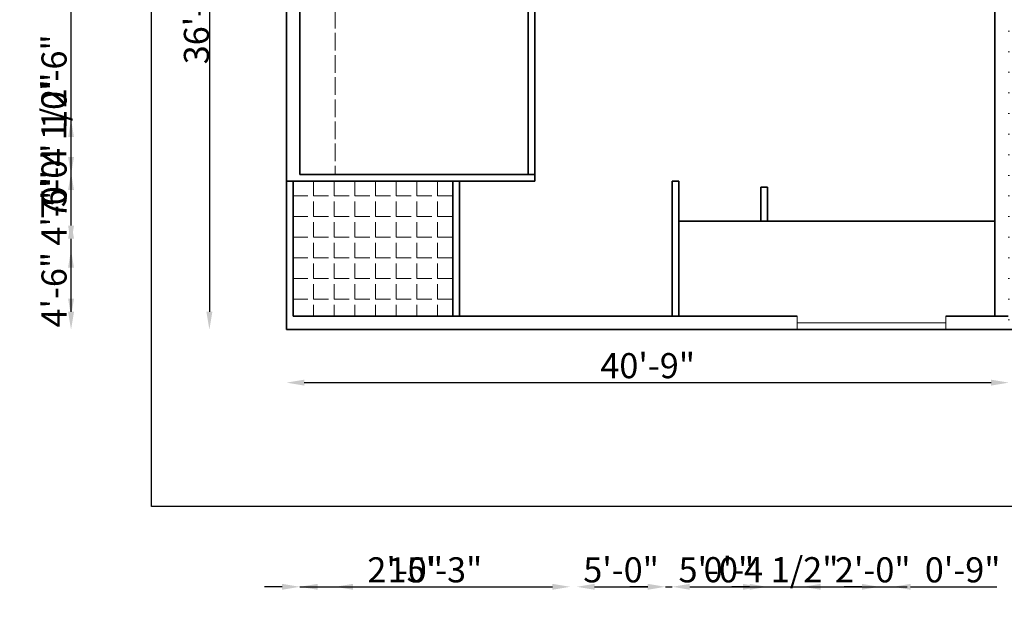
# Model space of a CAD drawing. Units: millimetres. Extents: x 1980 to 3220, y 1535 to 2343.
# Tile 1 of 3: x 1980 to 2647, y 1535 to 1936. Entities that reach past the tile are written whole.
import ezdxf

# ---------------------------------------------------------------- set-up
doc = ezdxf.new("R2010")
doc.units = ezdxf.units.MM
doc.linetypes.add('ACAD_ISO02W100', pattern=[15, 12, -3])
for name, color, linetype, lineweight in [('A-ANNO-DIMS', 2, 'Continuous', 18), ('A-FLOR-FIXT-OVHD', 9, 'ACAD_ISO02W100', 18), ('A-FLOR-PATT', 252, 'Continuous', 13), ('A-GLAZ', 4, 'Continuous', 18), ('A-WALL', 7, 'Continuous', 35), ('C-PROP', 8, 'Continuous', 25)]:
    doc.layers.add(name, color=color, linetype=linetype, lineweight=lineweight)
doc.styles.get("Standard").update_dxf_attribs({"font": 'arial.ttf'})
doc.dimstyles.new('ISO-25', dxfattribs={"dimtxt": 17, "dimasz": 12, "dimexe": 1.25, "dimexo": 0.625, "dimtad": 1, "dimdec": 1, "dimlunit": 4, "dimtxsty": 'Standard', "dimcen": 2.5, "dimse1": 1, "dimse2": 1, "dimadec": 0, "dimazin": 0, "dimtfac": 1, "dimtdec": 1, "dimtmove": 0, "dimatfit": 3, "dimfxl": 1, "dimarcsym": 0})

# ---------------------------------------------------------------- blocks, each defined once
blk = doc.blocks.new('*D4')
at = {"layer": 'A-ANNO-DIMS', "color": 0, "lineweight": -2, "transparency": 16777216}
blk.add_line((2173.01, 1689.61), (2638.01, 1689.61), dxfattribs=at)
at = {"layer": 'A-ANNO-DIMS', "color": 0, "transparency": 16777216}
for points in [[(2173.01, 1691.61), (2173.01, 1687.61), (2161.01, 1689.61)], [(2638.01, 1691.61), (2638.01, 1687.61), (2650.01, 1689.61)]]:
    blk.add_solid(points, dxfattribs=at)
at = {"layer": 'Defpoints', "color": 0, "transparency": 16777216}
for p in [(2161.01, 1725.6), (2650.01, 1725.6), (2650.01, 1689.61)]:
    blk.add_point(p, dxfattribs=at)
at = {"layer": 'A-ANNO-DIMS', "color": 0, "transparency": 16777216, "insert": (2405.51, 1698.91), "char_height": 17, "attachment_point": 5}
blk.add_mtext('40\'-9"', dxfattribs=at)
blk = doc.blocks.new('*D8')
at = {"layer": 'A-ANNO-DIMS', "color": 0, "lineweight": -2, "transparency": 16777216}
blk.add_line((2108.81, 2150.1), (2108.81, 1737.6), dxfattribs=at)
at = {"layer": 'A-ANNO-DIMS', "color": 0, "transparency": 16777216}
for points in [[(2106.81, 2150.1), (2110.81, 2150.1), (2108.81, 2162.1)], [(2106.81, 1737.6), (2110.81, 1737.6), (2108.81, 1725.6)]]:
    blk.add_solid(points, dxfattribs=at)
at = {"layer": 'Defpoints', "color": 0, "transparency": 16777216}
for p in [(2161.01, 2162.1), (2108.81, 1725.6), (2161.01, 1725.6)]:
    blk.add_point(p, dxfattribs=at)
at = {"layer": 'A-ANNO-DIMS', "color": 0, "transparency": 16777216, "insert": (2088.13, 1943.85), "char_height": 17, "attachment_point": 5, "rotation": 90}
blk.add_mtext('36\'-4{\\H1x;\\S1/2;}"', dxfattribs=at)
blk = doc.blocks.new('*D11')
at = {"layer": 'A-ANNO-DIMS', "color": 0, "lineweight": -2, "transparency": 16777216}
blk.add_line((2182.01, 1551.25), (2341.01, 1551.25), dxfattribs=at)
at = {"layer": 'A-ANNO-DIMS', "color": 0, "transparency": 16777216}
for points in [[(2182.01, 1553.25), (2182.01, 1549.25), (2170.01, 1551.25)], [(2341.01, 1553.25), (2341.01, 1549.25), (2353.01, 1551.25)]]:
    blk.add_solid(points, dxfattribs=at)
at = {"layer": 'Defpoints', "color": 0, "transparency": 16777216}
for p in [(2170.01, 2153.1), (2353.01, 2153.1), (2353.01, 1551.25)]:
    blk.add_point(p, dxfattribs=at)
at = {"layer": 'A-ANNO-DIMS', "color": 0, "transparency": 16777216, "insert": (2261.51, 1560.56), "char_height": 17, "attachment_point": 5}
blk.add_mtext('15\'-3"', dxfattribs=at)
blk = doc.blocks.new('*D12')
at = {"layer": 'A-ANNO-DIMS', "color": 0, "lineweight": -2, "transparency": 16777216}
blk.add_line((2369.51, 1551.25), (2405.51, 1551.25), dxfattribs=at)
at = {"layer": 'A-ANNO-DIMS', "color": 0, "transparency": 16777216}
for points in [[(2369.51, 1553.25), (2369.51, 1549.25), (2357.51, 1551.25)], [(2405.51, 1553.25), (2405.51, 1549.25), (2417.51, 1551.25)]]:
    blk.add_solid(points, dxfattribs=at)
at = {"layer": 'Defpoints', "color": 0, "transparency": 16777216}
for p in [(2357.51, 2153.1), (2417.51, 2153.1), (2417.51, 1551.25)]:
    blk.add_point(p, dxfattribs=at)
at = {"layer": 'A-ANNO-DIMS', "color": 0, "transparency": 16777216, "insert": (2387.51, 1560.55), "char_height": 17, "attachment_point": 5}
blk.add_mtext('5\'-0"', dxfattribs=at)
blk = doc.blocks.new('*D13')
at = {"layer": 'A-ANNO-DIMS', "color": 0, "lineweight": -2, "transparency": 16777216}
blk.add_line((2434.01, 1551.25), (2470.01, 1551.25), dxfattribs=at)
at = {"layer": 'A-ANNO-DIMS', "color": 0, "transparency": 16777216}
for points in [[(2434.01, 1553.25), (2434.01, 1549.25), (2422.01, 1551.25)], [(2470.01, 1553.25), (2470.01, 1549.25), (2482.01, 1551.25)]]:
    blk.add_solid(points, dxfattribs=at)
at = {"layer": 'Defpoints', "color": 0, "transparency": 16777216}
for p in [(2422.01, 2153.1), (2482.01, 2153.1), (2482.01, 1551.25)]:
    blk.add_point(p, dxfattribs=at)
at = {"layer": 'A-ANNO-DIMS', "color": 0, "transparency": 16777216, "insert": (2452.01, 1560.55), "char_height": 17, "attachment_point": 5}
blk.add_mtext('5\'-0"', dxfattribs=at)
blk = doc.blocks.new('*D17')
at = {"layer": 'A-ANNO-DIMS', "color": 0, "lineweight": -2, "transparency": 16777216}
blk.add_line((2182.01, 2307.95), (2312.51, 2307.95), dxfattribs=at)
at = {"layer": 'A-ANNO-DIMS', "color": 0, "transparency": 16777216}
for points in [[(2182.01, 2309.95), (2182.01, 2305.95), (2170.01, 2307.95)], [(2312.51, 2309.95), (2312.51, 2305.95), (2324.51, 2307.95)]]:
    blk.add_solid(points, dxfattribs=at)
at = {"layer": 'Defpoints', "color": 0, "transparency": 16777216}
for p in [(2324.51, 2307.95), (2170.01, 1830.6), (2324.51, 1830.6)]:
    blk.add_point(p, dxfattribs=at)
at = {"layer": 'A-ANNO-DIMS', "color": 0, "transparency": 16777216, "insert": (2247.26, 2317.36), "char_height": 17, "attachment_point": 5}
blk.add_mtext('12\'-10 1/2"', dxfattribs=at)
blk = doc.blocks.new('*D18')
at = {"layer": 'A-ANNO-DIMS', "color": 0, "lineweight": -2, "transparency": 16777216}
blk.add_line((2015.16, 1842.6), (2015.16, 1944.6), dxfattribs=at)
at = {"layer": 'A-ANNO-DIMS', "color": 0, "transparency": 16777216}
for points in [[(2013.16, 1944.6), (2017.16, 1944.6), (2015.16, 1956.6)], [(2013.16, 1842.6), (2017.16, 1842.6), (2015.16, 1830.6)]]:
    blk.add_solid(points, dxfattribs=at)
at = {"layer": 'Defpoints', "color": 0, "transparency": 16777216}
for p in [(2015.16, 1956.6), (2324.51, 1956.6), (2324.51, 1830.6)]:
    blk.add_point(p, dxfattribs=at)
at = {"layer": 'A-ANNO-DIMS', "color": 0, "transparency": 16777216, "insert": (2005.85, 1893.6), "char_height": 17, "attachment_point": 5, "rotation": 90}
blk.add_mtext('10\'-6"', dxfattribs=at)
blk = doc.blocks.new('*D25')
at = {"layer": 'A-ANNO-DIMS', "color": 0, "lineweight": -2, "transparency": 16777216}
blk.add_line((2177.51, 2307.95), (2261.51, 2307.95), dxfattribs=at)
at = {"layer": 'A-ANNO-DIMS', "color": 0, "transparency": 16777216}
for points in [[(2177.51, 2309.95), (2177.51, 2305.95), (2165.51, 2307.95)], [(2261.51, 2309.95), (2261.51, 2305.95), (2273.51, 2307.95)]]:
    blk.add_solid(points, dxfattribs=at)
at = {"layer": 'Defpoints', "color": 0, "transparency": 16777216}
for p in [(2273.51, 2307.95), (2165.51, 1734.6), (2273.51, 1734.6)]:
    blk.add_point(p, dxfattribs=at)
at = {"layer": 'A-ANNO-DIMS', "color": 0, "transparency": 16777216, "insert": (2219.51, 2317.25), "char_height": 17, "attachment_point": 5}
blk.add_mtext('9\'-0"', dxfattribs=at)
blk = doc.blocks.new('*D26')
at = {"layer": 'A-ANNO-DIMS', "color": 0, "lineweight": -2, "transparency": 16777216}
blk.add_line((2290.01, 2307.95), (2410.01, 2307.95), dxfattribs=at)
at = {"layer": 'A-ANNO-DIMS', "color": 0, "transparency": 16777216}
for points in [[(2290.01, 2309.95), (2290.01, 2305.95), (2278.01, 2307.95)], [(2410.01, 2309.95), (2410.01, 2305.95), (2422.01, 2307.95)]]:
    blk.add_solid(points, dxfattribs=at)
at = {"layer": 'Defpoints', "color": 0, "transparency": 16777216}
for p in [(2422.01, 2307.95), (2278.01, 1734.6), (2422.01, 1734.6)]:
    blk.add_point(p, dxfattribs=at)
at = {"layer": 'A-ANNO-DIMS', "color": 0, "transparency": 16777216, "insert": (2350.01, 2317.25), "char_height": 17, "attachment_point": 5}
blk.add_mtext('12\'-0"', dxfattribs=at)
blk = doc.blocks.new('*D27')
at = {"layer": 'A-ANNO-DIMS', "color": 0, "lineweight": -2, "transparency": 16777216}
blk.add_line((3203.86, 1746.6), (3203.86, 1814.1), dxfattribs=at)
at = {"layer": 'A-ANNO-DIMS', "color": 0, "transparency": 16777216}
for points in [[(3201.86, 1814.1), (3205.86, 1814.1), (3203.86, 1826.1)], [(3201.86, 1746.6), (3205.86, 1746.6), (3203.86, 1734.6)]]:
    blk.add_solid(points, dxfattribs=at)
at = {"layer": 'Defpoints', "color": 0, "transparency": 16777216}
for p in [(2278.01, 1826.1), (3203.86, 1826.1), (2278.01, 1734.6)]:
    blk.add_point(p, dxfattribs=at)
at = {"layer": 'A-ANNO-DIMS', "color": 0, "transparency": 16777216, "insert": (3194.44, 1780.35), "char_height": 17, "attachment_point": 5, "rotation": 90}
blk.add_mtext('7\'-7 1/2"', dxfattribs=at)
blk = doc.blocks.new('*D28')
at = {"layer": 'A-ANNO-DIMS', "color": 0, "lineweight": -2, "transparency": 16777216}
for p, q in [((2015.16, 1799.1), (2015.16, 1897.15)), ((2015.16, 1746.6), (2015.16, 1787.1))]:
    blk.add_line(p, q, dxfattribs=at)
at = {"layer": 'A-ANNO-DIMS', "color": 0, "transparency": 16777216}
for points in [[(2013.16, 1787.1), (2017.16, 1787.1), (2015.16, 1799.1)], [(2013.16, 1746.6), (2017.16, 1746.6), (2015.16, 1734.6)]]:
    blk.add_solid(points, dxfattribs=at)
at = {"layer": 'Defpoints', "color": 0, "transparency": 16777216}
for p in [(2015.16, 1799.1), (2640.51, 1799.1), (2640.51, 1734.6)]:
    blk.add_point(p, dxfattribs=at)
at = {"layer": 'A-ANNO-DIMS', "color": 0, "transparency": 16777216, "insert": (2005.74, 1854.12), "char_height": 17, "attachment_point": 5, "rotation": 90}
blk.add_mtext('5\'-4 1/2"', dxfattribs=at)
blk = doc.blocks.new('*D29')
at = {"layer": 'A-ANNO-DIMS', "color": 0, "lineweight": -2, "transparency": 16777216}
blk.add_line((2518.6, 2307.95), (2595.26, 2307.95), dxfattribs=at)
at = {"layer": 'A-ANNO-DIMS', "color": 0, "transparency": 16777216}
for points in [[(2518.6, 2309.95), (2518.6, 2305.95), (2506.6, 2307.95)], [(2595.26, 2309.95), (2595.26, 2305.95), (2607.26, 2307.95)]]:
    blk.add_solid(points, dxfattribs=at)
at = {"layer": 'Defpoints', "color": 0, "transparency": 16777216}
for p in [(2607.26, 2307.95), (2506.6, 1734.6), (2607.26, 1734.6)]:
    blk.add_point(p, dxfattribs=at)
at = {"layer": 'A-ANNO-DIMS', "color": 0, "transparency": 16777216, "insert": (2556.93, 2317.36), "char_height": 17, "attachment_point": 5}
blk.add_mtext('8\'-4 1/2"', dxfattribs=at)
blk = doc.blocks.new('*D30')
at = {"layer": 'A-ANNO-DIMS', "color": 0, "lineweight": -2, "transparency": 16777216}
for p, q in [((2619.26, 2307.95), (2628.51, 2307.95)), ((2640.51, 2307.95), (2738.85, 2307.95))]:
    blk.add_line(p, q, dxfattribs=at)
at = {"layer": 'A-ANNO-DIMS', "color": 0, "transparency": 16777216}
for points in [[(2619.26, 2309.95), (2619.26, 2305.95), (2607.26, 2307.95)], [(2628.51, 2309.95), (2628.51, 2305.95), (2640.51, 2307.95)]]:
    blk.add_solid(points, dxfattribs=at)
at = {"layer": 'Defpoints', "color": 0, "transparency": 16777216}
for p in [(2640.51, 2307.95), (2607.26, 1734.6), (2640.51, 1734.6)]:
    blk.add_point(p, dxfattribs=at)
at = {"layer": 'A-ANNO-DIMS', "color": 0, "transparency": 16777216, "insert": (2695.68, 2317.36), "char_height": 17, "attachment_point": 5}
blk.add_mtext('2\'-9 1/2"', dxfattribs=at)
blk = doc.blocks.new('*D42')
at = {"layer": 'A-ANNO-DIMS', "color": 0, "lineweight": -2, "transparency": 16777216}
blk.add_line((2015.16, 1796.1), (2015.16, 1856.1), dxfattribs=at)
at = {"layer": 'A-ANNO-DIMS', "color": 0, "transparency": 16777216}
for points in [[(2013.16, 1856.1), (2017.16, 1856.1), (2015.16, 1868.1)], [(2013.16, 1796.1), (2017.16, 1796.1), (2015.16, 1784.1)]]:
    blk.add_solid(points, dxfattribs=at)
at = {"layer": 'Defpoints', "color": 0, "transparency": 16777216}
for p in [(2015.16, 1868.1), (3049.01, 1868.1), (3049.01, 1784.1)]:
    blk.add_point(p, dxfattribs=at)
at = {"layer": 'A-ANNO-DIMS', "color": 0, "transparency": 16777216, "insert": (2005.85, 1826.1), "char_height": 17, "attachment_point": 5, "rotation": 90}
blk.add_mtext('7\'-0"', dxfattribs=at)
blk = doc.blocks.new('*D43')
at = {"layer": 'A-ANNO-DIMS', "color": 0, "lineweight": -2, "transparency": 16777216}
blk.add_line((2015.16, 1796.1), (2015.16, 1820.1), dxfattribs=at)
at = {"layer": 'A-ANNO-DIMS', "color": 0, "transparency": 16777216}
for points in [[(2013.16, 1820.1), (2017.16, 1820.1), (2015.16, 1832.1)], [(2013.16, 1796.1), (2017.16, 1796.1), (2015.16, 1784.1)]]:
    blk.add_solid(points, dxfattribs=at)
at = {"layer": 'Defpoints', "color": 0, "transparency": 16777216}
for p in [(2015.16, 1832.1), (2944.01, 1832.1), (2939.51, 1784.1)]:
    blk.add_point(p, dxfattribs=at)
at = {"layer": 'A-ANNO-DIMS', "color": 0, "transparency": 16777216, "insert": (2005.85, 1808.1), "char_height": 17, "attachment_point": 5, "rotation": 90}
blk.add_mtext('4\'-0"', dxfattribs=at)
blk = doc.blocks.new('*D44')
at = {"layer": 'A-ANNO-DIMS', "color": 0, "lineweight": -2, "transparency": 16777216}
blk.add_line((2015.16, 1737.6), (2015.16, 1767.6), dxfattribs=at)
at = {"layer": 'A-ANNO-DIMS', "color": 0, "transparency": 16777216}
for points in [[(2013.16, 1767.6), (2017.16, 1767.6), (2015.16, 1779.6)], [(2013.16, 1737.6), (2017.16, 1737.6), (2015.16, 1725.6)]]:
    blk.add_solid(points, dxfattribs=at)
at = {"layer": 'Defpoints', "color": 0, "transparency": 16777216}
for p in [(2015.16, 1779.6), (3058.01, 1779.6), (3058.01, 1725.6)]:
    blk.add_point(p, dxfattribs=at)
at = {"layer": 'A-ANNO-DIMS', "color": 0, "transparency": 16777216, "insert": (2005.85, 1752.6), "char_height": 17, "attachment_point": 5, "rotation": 90}
blk.add_mtext('4\'-6"', dxfattribs=at)
blk = doc.blocks.new('*D50')
at = {"layer": 'A-ANNO-DIMS', "color": 0, "lineweight": -2, "transparency": 16777216}
for p, q in [((2405.51, 1551.25), (2393.51, 1551.25)), ((2417.51, 1551.25), (2422.01, 1551.25)), ((2434.01, 1551.25), (2532.06, 1551.25))]:
    blk.add_line(p, q, dxfattribs=at)
at = {"layer": 'A-ANNO-DIMS', "color": 0, "transparency": 16777216}
for points in [[(2405.51, 1553.25), (2405.51, 1549.25), (2417.51, 1551.25)], [(2434.01, 1553.25), (2434.01, 1549.25), (2422.01, 1551.25)]]:
    blk.add_solid(points, dxfattribs=at)
at = {"layer": 'Defpoints', "color": 0, "transparency": 16777216}
for p in [(2417.51, 2063.1), (2422.01, 2063.1), (2422.01, 1551.25)]:
    blk.add_point(p, dxfattribs=at)
at = {"layer": 'A-ANNO-DIMS', "color": 0, "transparency": 16777216, "insert": (2489.03, 1560.66), "char_height": 17, "attachment_point": 5}
blk.add_mtext('0\'-4 1/2"', dxfattribs=at)
blk = doc.blocks.new('*D53')
at = {"layer": 'A-ANNO-DIMS', "color": 0, "lineweight": -2, "transparency": 16777216}
for p, q in [((2474.51, 1551.25), (2462.51, 1551.25)), ((2486.51, 1551.25), (2510.51, 1551.25)), ((2522.51, 1551.25), (2581.24, 1551.25))]:
    blk.add_line(p, q, dxfattribs=at)
at = {"layer": 'A-ANNO-DIMS', "color": 0, "transparency": 16777216}
for points in [[(2474.51, 1553.25), (2474.51, 1549.25), (2486.51, 1551.25)], [(2522.51, 1553.25), (2522.51, 1549.25), (2510.51, 1551.25)]]:
    blk.add_solid(points, dxfattribs=at)
at = {"layer": 'Defpoints', "color": 0, "transparency": 16777216}
for p in [(2486.51, 2086.35), (2510.51, 2086.35), (2510.51, 1551.25)]:
    blk.add_point(p, dxfattribs=at)
at = {"layer": 'A-ANNO-DIMS', "color": 0, "transparency": 16777216, "insert": (2557.87, 1560.55), "char_height": 17, "attachment_point": 5}
blk.add_mtext('2\'-0"', dxfattribs=at)
blk = doc.blocks.new('*D54')
at = {"layer": 'A-ANNO-DIMS', "color": 0, "lineweight": -2, "transparency": 16777216}
for p, q in [((2438.51, 2307.95), (2470.01, 2307.95)), ((2482.01, 2307.95), (2580.75, 2307.95))]:
    blk.add_line(p, q, dxfattribs=at)
at = {"layer": 'A-ANNO-DIMS', "color": 0, "transparency": 16777216}
for points in [[(2438.51, 2309.95), (2438.51, 2305.95), (2426.51, 2307.95)], [(2470.01, 2309.95), (2470.01, 2305.95), (2482.01, 2307.95)]]:
    blk.add_solid(points, dxfattribs=at)
at = {"layer": 'Defpoints', "color": 0, "transparency": 16777216}
for p in [(2482.01, 2307.95), (2426.51, 1799.1), (2482.01, 1799.1)]:
    blk.add_point(p, dxfattribs=at)
at = {"layer": 'A-ANNO-DIMS', "color": 0, "transparency": 16777216, "insert": (2537.38, 2317.36), "char_height": 17, "attachment_point": 5}
blk.add_mtext('4\'-7 1/2"', dxfattribs=at)
blk = doc.blocks.new('*D55')
at = {"layer": 'A-ANNO-DIMS', "color": 0, "lineweight": -2, "transparency": 16777216}
for p, q in [((3203.86, 1834.1), (3203.86, 1904.15)), ((3203.86, 1799.1), (3203.86, 1822.1)), ((3203.86, 1787.1), (3203.86, 1775.1))]:
    blk.add_line(p, q, dxfattribs=at)
at = {"layer": 'A-ANNO-DIMS', "color": 0, "transparency": 16777216}
for points in [[(3201.86, 1834.1), (3205.86, 1834.1), (3203.86, 1822.1)], [(3201.86, 1787.1), (3205.86, 1787.1), (3203.86, 1799.1)]]:
    blk.add_solid(points, dxfattribs=at)
at = {"layer": 'Defpoints', "color": 0, "transparency": 16777216}
for p in [(2482.01, 1822.1), (3203.86, 1822.1), (2482.01, 1799.1)]:
    blk.add_point(p, dxfattribs=at)
at = {"layer": 'A-ANNO-DIMS', "color": 0, "transparency": 16777216, "insert": (3194.7, 1875.12), "char_height": 17, "attachment_point": 5, "rotation": 90}
blk.add_mtext('1\'-11"', dxfattribs=at)
blk = doc.blocks.new('*D56')
at = {"layer": 'A-ANNO-DIMS', "color": 0, "lineweight": -2, "transparency": 16777216}
for p, q in [((2158.01, 1551.25), (2146.01, 1551.25)), ((2170.01, 1551.25), (2194.01, 1551.25)), ((2206.01, 1551.25), (2264.74, 1551.25))]:
    blk.add_line(p, q, dxfattribs=at)
at = {"layer": 'A-ANNO-DIMS', "color": 0, "transparency": 16777216}
for points in [[(2158.01, 1553.25), (2158.01, 1549.25), (2170.01, 1551.25)], [(2206.01, 1553.25), (2206.01, 1549.25), (2194.01, 1551.25)]]:
    blk.add_solid(points, dxfattribs=at)
at = {"layer": 'Defpoints', "color": 0, "transparency": 16777216}
for p in [(2170.01, 1830.6), (2194.01, 1830.6), (2194.01, 1551.25)]:
    blk.add_point(p, dxfattribs=at)
at = {"layer": 'A-ANNO-DIMS', "color": 0, "transparency": 16777216, "insert": (2241.37, 1560.55), "char_height": 17, "attachment_point": 5}
blk.add_mtext('2\'-0"', dxfattribs=at)
blk = doc.blocks.new('*D57')
at = {"layer": 'A-ANNO-DIMS', "color": 0, "lineweight": -2, "transparency": 16777216}
for p, q in [((2550.51, 1551.25), (2538.51, 1551.25)), ((2562.51, 1551.25), (2571.51, 1551.25)), ((2583.51, 1551.25), (2641.95, 1551.25))]:
    blk.add_line(p, q, dxfattribs=at)
at = {"layer": 'A-ANNO-DIMS', "color": 0, "transparency": 16777216}
for points in [[(2550.51, 1553.25), (2550.51, 1549.25), (2562.51, 1551.25)], [(2583.51, 1553.25), (2583.51, 1549.25), (2571.51, 1551.25)]]:
    blk.add_solid(points, dxfattribs=at)
at = {"layer": 'Defpoints', "color": 0, "transparency": 16777216}
for p in [(2562.51, 1946.1), (2571.51, 1946.1), (2571.51, 1551.25)]:
    blk.add_point(p, dxfattribs=at)
at = {"layer": 'A-ANNO-DIMS', "color": 0, "transparency": 16777216, "insert": (2618.73, 1560.55), "char_height": 17, "attachment_point": 5}
blk.add_mtext('0\'-9"', dxfattribs=at)

msp = doc.modelspace()

# ---------------------------------------------------------------- hatches: boundary and pattern name
at = {"layer": 'A-FLOR-PATT'}
h = msp.add_hatch(dxfattribs=at)
h.set_pattern_fill('ANGLE', color=256, scale=2)
h.set_pattern_definition([(0, (0, 0), (0, 13.97), [10.16, -3.81]), (90, (0, 0), (-13.97, 9e-16), [10.16, -3.81])])
h.paths.add_polyline_path([(2727.51, 1988.82), (2688.51, 1988.82), (2688.51, 2036.82), (2649.51, 2036.82), (2649.51, 1725.6), (2727.51, 1725.6)])
h.paths.add_polyline_path([(2273.51, 1826.1), (2165.51, 1826.1), (2165.51, 1734.6), (2273.51, 1734.6)])

# ---------------------------------------------------------------- linework, layer by layer
at = {"layer": 'A-FLOR-FIXT-OVHD'}
msp.add_line((2194.01, 1956.6), (2194.01, 1830.6), dxfattribs=at)
at = {"layer": 'A-GLAZ'}
for p, q in [((2506.6, 1734.6), (2506.6, 1725.6)), ((2607.26, 1734.6), (2607.26, 1725.6)), ((2607.26, 1730.1), (2506.6, 1730.1))]:
    msp.add_line(p, q, dxfattribs=at)
at = {"layer": 'A-WALL'}
for p, q in [((2161.01, 1725.6), (2161.01, 2162.1)), ((2170.01, 1830.6), (2170.01, 2153.1)), ((2640.51, 1734.6), (2640.51, 2153.1)), ((2324.51, 1956.6), (2324.51, 1830.6)), ((2329.01, 1956.6), (2329.01, 1826.1)), ((2170.01, 1830.6), (2329.01, 1830.6)), ((2161.01, 1826.1), (2329.01, 1826.1)), ((2165.51, 1734.6), (2165.51, 1826.1)), ((2273.51, 1734.6), (2273.51, 1826.1)), ((2278.01, 1734.6), (2278.01, 1826.1)), ((2422.01, 1734.6), (2422.01, 1826.1)), ((2426.51, 1826.1), (2422.01, 1826.1)), ((2426.51, 1734.6), (2426.51, 1826.1)), ((2482.01, 1799.1), (2482.01, 1822.1)), ((2486.51, 1822.1), (2482.01, 1822.1)), ((2486.51, 1799.1), (2486.51, 1822.1)), ((2426.51, 1799.1), (2640.51, 1799.1)), ((2506.6, 1734.6), (2165.51, 1734.6)), ((2649.51, 1734.6), (2607.26, 1734.6)), ((3058.01, 1725.6), (2161.01, 1725.6))]:
    msp.add_line(p, q, dxfattribs=at)
at = {"layer": 'C-PROP'}
msp.add_line((2069.51, 1929.6), (2069.51, 1929.6), dxfattribs=at)
msp.add_lwpolyline([(2069.51, 2253.6), (3149.51, 2253.6), (3149.51, 1605.6), (2069.51, 1605.6)], close=True, dxfattribs=at)

# ---------------------------------------------------------------- dimensions: what is measured, and where the dimension line sits
at = {"layer": 'A-ANNO-DIMS'}
for base, p1, p2, override, picture, middle in [((2324.51, 2307.95), (2170.01, 1830.6), (2324.51, 1830.6), {"dimdec": 1, "dimlfac": 1, "dimrnd": 0, "dimzin": 1, "dimdsep": 46, "dimlunit": 4, "dimfrac": 2}, '*D17', (2247.26, 2317.36)), ((2482.01, 2307.95), (2426.51, 1799.1), (2482.01, 1799.1), {"dimdec": 1, "dimlfac": 1, "dimrnd": 0, "dimzin": 1, "dimdsep": 46, "dimlunit": 4, "dimfrac": 2}, '*D54', (2537.38, 2317.36)), ((2607.26, 2307.95), (2506.6, 1734.6), (2607.26, 1734.6), {"dimdec": 1, "dimlfac": 1, "dimrnd": 0, "dimzin": 1, "dimdsep": 46, "dimlunit": 4, "dimfrac": 2}, '*D29', (2556.93, 2317.36)), ((2640.508481, 2307.945639), (2607.258481, 1734.595639), (2640.508481, 1734.595639), {"dimdec": 1, "dimlfac": 1, "dimrnd": 0, "dimzin": 1, "dimdsep": 46, "dimlunit": 4, "dimfrac": 2}, '*D30', (2695.67986572, 2317.3605435)), ((2273.51, 2307.95), (2165.51, 1734.6), (2273.51, 1734.6), {"dimdec": 1, "dimlfac": 1, "dimrnd": 0, "dimzin": 1, "dimdsep": 46, "dimlunit": 4, "dimfrac": 2}, '*D25', (2219.51, 2317.25)), ((2422.01, 2307.95), (2278.01, 1734.6), (2422.01, 1734.6), {"dimdec": 1, "dimlfac": 1, "dimrnd": 0, "dimzin": 1, "dimdsep": 46, "dimlunit": 4, "dimfrac": 2}, '*D26', (2350.01, 2317.25)), ((2353.01, 1551.25), (2170.01, 2153.1), (2353.01, 2153.1), {"dimdec": 1, "dimlfac": 1, "dimrnd": 0, "dimzin": 1, "dimdsep": 46, "dimlunit": 4, "dimfrac": 2}, '*D11', (2261.51, 1560.56)), ((2417.51, 1551.25), (2357.51, 2153.1), (2417.51, 2153.1), {"dimdec": 1, "dimlfac": 1, "dimrnd": 0, "dimzin": 1, "dimdsep": 46, "dimlunit": 4, "dimfrac": 2}, '*D12', (2387.51, 1560.55)), ((2482.01, 1551.25), (2422.01, 2153.1), (2482.01, 2153.1), {"dimdec": 1, "dimlfac": 1, "dimrnd": 0, "dimzin": 1, "dimdsep": 46, "dimlunit": 4, "dimfrac": 2}, '*D13', (2452.01, 1560.55)), ((2510.51, 1551.25), (2486.51, 2086.35), (2510.51, 2086.35), {"dimdec": 1, "dimlfac": 1, "dimrnd": 0, "dimzin": 1, "dimdsep": 46, "dimlunit": 4, "dimfrac": 2}, '*D53', (2557.87, 1560.55)), ((2422.01, 1551.25), (2417.51, 2063.1), (2422.01, 2063.1), {"dimdec": 1, "dimlfac": 1, "dimrnd": 0, "dimzin": 1, "dimdsep": 46, "dimlunit": 4, "dimfrac": 2}, '*D50', (2489.03, 1560.66)), ((2571.51, 1551.25), (2562.51, 1946.1), (2571.51, 1946.1), {"dimdec": 1, "dimlfac": 1, "dimrnd": 0, "dimzin": 1, "dimdsep": 46, "dimlunit": 4, "dimfrac": 2}, '*D57', (2618.73, 1560.55)), ((2194.01, 1551.25), (2170.01, 1830.6), (2194.01, 1830.6), {"dimdec": 1, "dimlfac": 1, "dimrnd": 0, "dimzin": 1, "dimdsep": 46, "dimlunit": 4, "dimfrac": 2}, '*D56', (2241.37, 1560.55)), ((2650.01, 1689.61), (2161.01, 1725.6), (2650.01, 1725.6), {"dimclrd": 0, "dimclre": 0, "dimclrt": 0}, '*D4', (2405.51, 1698.91))]:
    dim = msp.add_linear_dim(base=base, p1=p1, p2=p2, dimstyle='ISO-25', override=override, dxfattribs=at)
    dim.commit()
    dim.dimension.update_dxf_attribs({"geometry": picture, "text_midpoint": middle})
for base, p1, p2, override, picture, middle in [((2108.81, 1725.6), (2161.01, 2162.1), (2161.01, 1725.6), {"dimclrd": 0, "dimclre": 0, "dimclrt": 0}, '*D8', (2088.13, 1943.85)), ((2015.16, 1956.6), (2324.51, 1830.6), (2324.51, 1956.6), {"dimdec": 1, "dimlfac": 1, "dimrnd": 0, "dimzin": 1, "dimdsep": 46, "dimlunit": 4, "dimfrac": 2}, '*D18', (2005.85, 1893.6)), ((3203.86, 1822.1), (2482.01, 1799.1), (2482.01, 1822.1), {"dimdec": 1, "dimlfac": 1, "dimrnd": 0, "dimzin": 1, "dimdsep": 46, "dimlunit": 4, "dimfrac": 2}, '*D55', (3194.7, 1875.12)), ((2015.16, 1799.1), (2640.51, 1734.6), (2640.51, 1799.1), {"dimdec": 1, "dimlfac": 1, "dimrnd": 0, "dimzin": 1, "dimdsep": 46, "dimlunit": 4, "dimfrac": 2}, '*D28', (2005.74, 1854.12)), ((2015.16, 1868.1), (3049.01, 1784.1), (3049.01, 1868.1), {"dimdec": 1, "dimlfac": 1, "dimrnd": 0, "dimzin": 1, "dimdsep": 46, "dimlunit": 4, "dimfrac": 2}, '*D42', (2005.85, 1826.1)), ((2015.16, 1832.1), (2939.51, 1784.1), (2944.01, 1832.1), {"dimdec": 1, "dimlfac": 1, "dimrnd": 0, "dimzin": 1, "dimdsep": 46, "dimlunit": 4, "dimfrac": 2}, '*D43', (2005.85, 1808.1)), ((3203.86, 1826.1), (2278.01, 1734.6), (2278.01, 1826.1), {"dimdec": 1, "dimlfac": 1, "dimrnd": 0, "dimzin": 1, "dimdsep": 46, "dimlunit": 4, "dimfrac": 2}, '*D27', (3194.44, 1780.35)), ((2015.16, 1779.6), (3058.01, 1725.6), (3058.01, 1779.6), {"dimdec": 1, "dimlfac": 1, "dimrnd": 0, "dimzin": 1, "dimdsep": 46, "dimlunit": 4, "dimfrac": 2}, '*D44', (2005.85, 1752.6))]:
    dim = msp.add_linear_dim(base=base, p1=p1, p2=p2, angle=90, dimstyle='ISO-25', override=override, dxfattribs=at)
    dim.commit()
    dim.dimension.update_dxf_attribs({"geometry": picture, "text_midpoint": middle})

doc.saveas('drawing.dxf')
